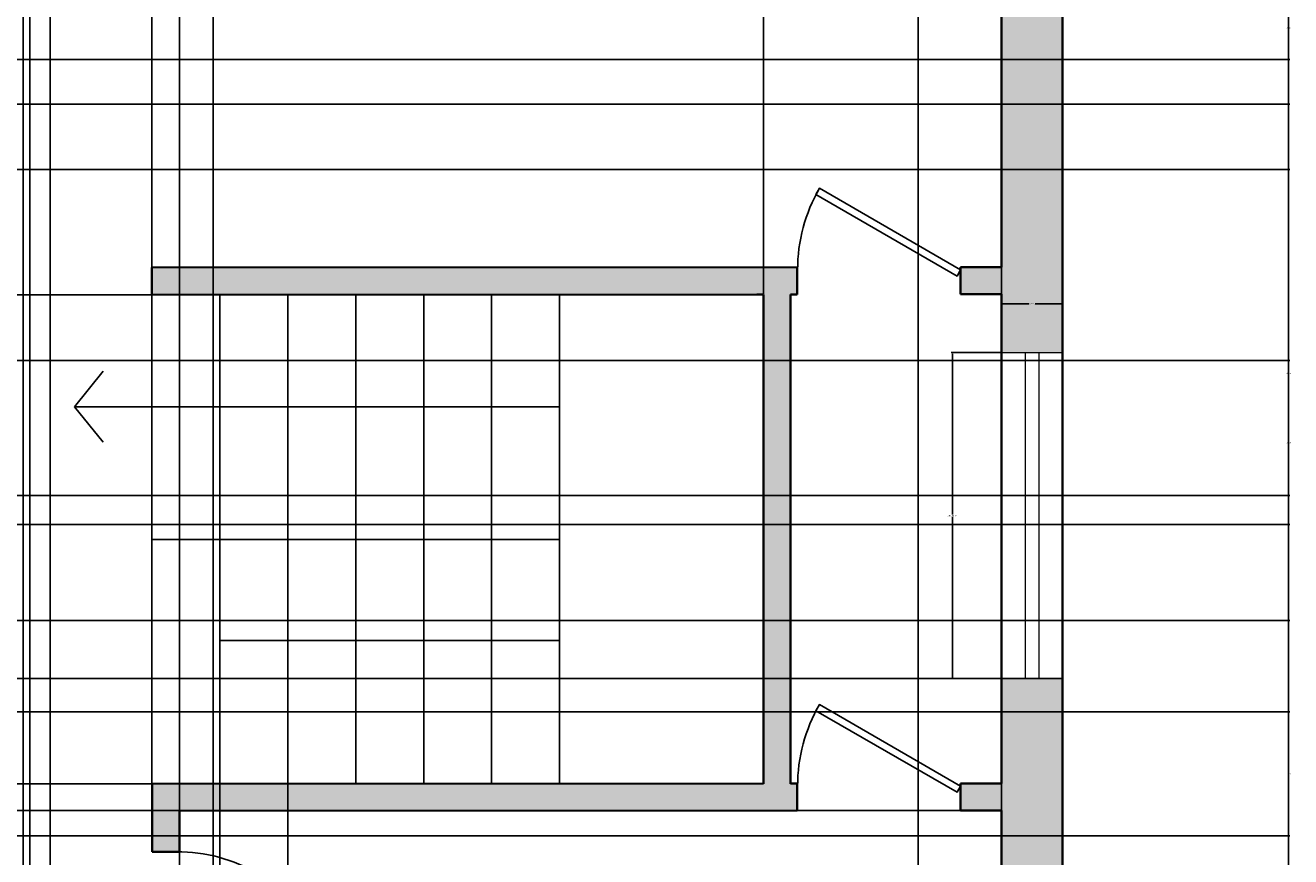
# Model space of a CAD drawing. Units: inches. Extents: x 1531 to 2263, y 2711 to 3216.
# Tile 10 of 12: x 2076 to 2262, y 2893 to 3015. Entities that reach past the tile are written whole.
import ezdxf

# ---------------------------------------------------------------- set-up
doc = ezdxf.new("R2010")
doc.units = ezdxf.units.IN
for name, color, linetype, lineweight in [('A-ANNO-DIMS', 2, 'Continuous', 18), ('A-DOOR', 3, 'Continuous', 25), ('A-FLOR-STRS', 7, 'Continuous', 25), ('A-GLAZ', 4, 'Continuous', 18), ('A-WALL', 7, 'Continuous', 35)]:
    doc.layers.add(name, color=color, linetype=linetype, lineweight=lineweight)
doc.layers.add('A-WALL-PATT', color=18, linetype='Continuous', lineweight=13, true_color=0x000000)
doc.styles.get("Standard").update_dxf_attribs({"font": 'arial.ttf'})
doc.dimstyles.get("Standard").update_dxf_attribs({"dimtxt": 0.18, "dimasz": 0.18, "dimexe": 0.18, "dimexo": 0.0625, "dimgap": 0.09, "dimtad": 0, "dimtih": 1, "dimtoh": 1, "dimdec": 4, "dimzin": 0, "dimdsep": 46, "dimtxsty": 'Standard', "dimcen": 0.09, "dimadec": 0, "dimazin": 0, "dimtfac": 1, "dimtdec": 4, "dimtofl": 0, "dimtmove": 0, "dimatfit": 3, "dimfxl": 1, "dimtolj": 1, "dimtzin": 0, "dimarcsym": 0})

# ---------------------------------------------------------------- blocks, each defined once
blk = doc.blocks.new('*U3')
for p, q in [((0, 0), (0, -6)), ((40, 0), (40, -6))]:
    blk.add_line(p, q)
blk.add_lwpolyline([(0, 0), (34.64, 20), (35.52, 18.48), (0.87, -1.52)], close=True)
blk.add_arc((0, 0), 40, 0, 30)
blk = doc.blocks.new('WIN-48IN')
for p, q in [((3.5, 48), (3.5, 0)), ((5.5, 48), (5.5, 0))]:
    blk.add_line(p, q)
for points in [[(0, 48), (9, 48)], [(9, 0), (0, 0)]]:
    blk.add_lwpolyline(points)
blk = doc.blocks.new('*D30')
at = {"layer": 'A-ANNO-DIMS', "color": 0, "lineweight": -2, "transparency": 16777216}
for p, q in [((2219.85, 2966.81), (2212.53, 2966.81)), ((2212.71, 2966.63), (2212.71, 2942.99)), ((2212.71, 2918.99), (2212.71, 2942.62)), ((2219.85, 2918.81), (2212.53, 2918.81))]:
    blk.add_line(p, q, dxfattribs=at)
at = {"layer": 'A-ANNO-DIMS', "color": 0, "transparency": 16777216}
for points in [[(2212.68, 2966.63), (2212.74, 2966.63), (2212.71, 2966.81)], [(2212.68, 2918.99), (2212.74, 2918.99), (2212.71, 2918.81)]]:
    blk.add_solid(points, dxfattribs=at)
at = {"layer": 'Defpoints', "color": 0, "transparency": 16777216}
for p in [(2212.71, 2966.81), (2219.91, 2966.81), (2219.91, 2918.81)]:
    blk.add_point(p, dxfattribs=at)
at = {"layer": 'A-ANNO-DIMS', "color": 0, "transparency": 16777216, "insert": (2212.71, 2942.81), "char_height": 0.18, "attachment_point": 5}
blk.add_mtext('\\A1;WDW 48 TYP.', dxfattribs=at)
blk = doc.blocks.new('*D31')
at = {"layer": 'A-ANNO-DIMS', "color": 0, "lineweight": -2, "transparency": 16777216}
for p, q in [((2219.91, 2966.87), (2219.91, 2974.19)), ((2220.09, 2974.01), (2223.95, 2974.01)), ((2228.73, 2974.01), (2224.87, 2974.01)), ((2228.91, 2966.87), (2228.91, 2974.19))]:
    blk.add_line(p, q, dxfattribs=at)
at = {"layer": 'A-ANNO-DIMS', "color": 0, "transparency": 16777216}
for points in [[(2220.09, 2974.04), (2220.09, 2973.98), (2219.91, 2974.01)], [(2228.73, 2974.04), (2228.73, 2973.98), (2228.91, 2974.01)]]:
    blk.add_solid(points, dxfattribs=at)
at = {"layer": 'Defpoints', "color": 0, "transparency": 16777216}
for p in [(2228.91, 2974.01), (2219.91, 2966.81), (2228.91, 2966.81)]:
    blk.add_point(p, dxfattribs=at)
at = {"layer": 'A-ANNO-DIMS', "color": 0, "transparency": 16777216, "insert": (2224.41, 2974.01), "char_height": 0.18, "attachment_point": 5}
blk.add_mtext('\\A1;9 TYP.', dxfattribs=at)
blk = doc.blocks.new('*D55')
at = {"layer": 'A-ANNO-DIMS', "color": 0, "lineweight": -2, "transparency": 16777216}
for p, q in [((2228.97, 3183.02), (2262.37, 3183.02)), ((2262.19, 3182.84), (2262.19, 2963.95)), ((2262.19, 2744.7), (2262.19, 2963.59)), ((2076.3, 2744.52), (2262.37, 2744.52))]:
    blk.add_line(p, q, dxfattribs=at)
at = {"layer": 'A-ANNO-DIMS', "color": 0, "transparency": 16777216}
for points in [[(2262.16, 3182.84), (2262.22, 3182.84), (2262.19, 3183.02)], [(2262.16, 2744.7), (2262.22, 2744.7), (2262.19, 2744.52)]]:
    blk.add_solid(points, dxfattribs=at)
at = {"layer": 'Defpoints', "color": 0, "transparency": 16777216}
for p in [(2228.91, 3183.02), (2076.24, 2744.52), (2262.19, 2744.52)]:
    blk.add_point(p, dxfattribs=at)
at = {"layer": 'A-ANNO-DIMS', "color": 0, "transparency": 16777216, "insert": (2262.19, 2963.77), "char_height": 0.18, "attachment_point": 5}
blk.add_mtext('\\A1;438.5', dxfattribs=at)
blk = doc.blocks.new('*D74')
at = {"layer": 'A-ANNO-DIMS', "color": 0, "lineweight": -2, "transparency": 16777216}
for p, q in [((2098.91, 2899.27), (2098.91, 2711.06)), ((2219.91, 2899.33), (2219.91, 2711.06)), ((2099.09, 2711.24), (2159.15, 2711.24)), ((2219.73, 2711.24), (2159.67, 2711.24))]:
    blk.add_line(p, q, dxfattribs=at)
at = {"layer": 'A-ANNO-DIMS', "color": 0, "transparency": 16777216}
for points in [[(2099.09, 2711.27), (2099.09, 2711.21), (2098.91, 2711.24)], [(2219.73, 2711.27), (2219.73, 2711.21), (2219.91, 2711.24)]]:
    blk.add_solid(points, dxfattribs=at)
at = {"layer": 'Defpoints', "color": 0, "transparency": 16777216}
for p in [(2098.91, 2899.33), (2219.91, 2899.4), (2219.91, 2711.24)]:
    blk.add_point(p, dxfattribs=at)
at = {"layer": 'A-ANNO-DIMS', "color": 0, "transparency": 16777216, "insert": (2159.41, 2711.24), "char_height": 0.18, "attachment_point": 5}
blk.add_mtext('\\A1;121', dxfattribs=at)
blk = doc.blocks.new('*D75')
at = {"layer": 'A-ANNO-DIMS', "color": 0, "lineweight": -2, "transparency": 16777216}
for p, q in [((2219.85, 2899.4), (1531.04, 2899.4)), ((1531.22, 2899.22), (1531.22, 2853.81)), ((1531.22, 2808.04), (1531.22, 2853.45)), ((2219.85, 2807.86), (1531.04, 2807.86))]:
    blk.add_line(p, q, dxfattribs=at)
at = {"layer": 'A-ANNO-DIMS', "color": 0, "transparency": 16777216}
for points in [[(1531.19, 2899.22), (1531.25, 2899.22), (1531.22, 2899.4)], [(1531.19, 2808.04), (1531.25, 2808.04), (1531.22, 2807.86)]]:
    blk.add_solid(points, dxfattribs=at)
at = {"layer": 'Defpoints', "color": 0, "transparency": 16777216}
for p in [(1531.22, 2899.4), (2219.91, 2899.4), (2219.91, 2807.86)]:
    blk.add_point(p, dxfattribs=at)
at = {"layer": 'A-ANNO-DIMS', "color": 0, "transparency": 16777216, "insert": (1531.22, 2853.63), "char_height": 0.18, "attachment_point": 5}
blk.add_mtext('\\A1;91.53', dxfattribs=at)
blk = doc.blocks.new('*D76')
at = {"layer": 'A-ANNO-DIMS', "color": 0, "lineweight": -2, "transparency": 16777216}
for p, q in [((2094.87, 2975.39), (2094.87, 3216.47)), ((2095.05, 3216.29), (2139.65, 3216.29)), ((2184.69, 3216.29), (2140.09, 3216.29)), ((2184.87, 2975.44), (2184.87, 3216.47))]:
    blk.add_line(p, q, dxfattribs=at)
at = {"layer": 'A-ANNO-DIMS', "color": 0, "transparency": 16777216}
for points in [[(2095.05, 3216.32), (2095.05, 3216.26), (2094.87, 3216.29)], [(2184.69, 3216.32), (2184.69, 3216.26), (2184.87, 3216.29)]]:
    blk.add_solid(points, dxfattribs=at)
at = {"layer": 'Defpoints', "color": 0, "transparency": 16777216}
for p in [(2184.87, 3216.29), (2094.87, 2975.33), (2184.87, 2975.38)]:
    blk.add_point(p, dxfattribs=at)
at = {"layer": 'A-ANNO-DIMS', "color": 0, "transparency": 16777216, "insert": (2139.87, 3216.29), "char_height": 0.18, "attachment_point": 5}
blk.add_mtext('\\A1;90', dxfattribs=at)
blk = doc.blocks.new('*D77')
at = {"layer": 'A-ANNO-DIMS', "color": 0, "lineweight": -2, "transparency": 16777216}
for p, q in [((2094.81, 2975.33), (1531.04, 2975.33)), ((1531.22, 2975.15), (1531.22, 2939.52)), ((1531.22, 2903.53), (1531.22, 2939.16)), ((2094.81, 2903.35), (1531.04, 2903.35))]:
    blk.add_line(p, q, dxfattribs=at)
at = {"layer": 'A-ANNO-DIMS', "color": 0, "transparency": 16777216}
for points in [[(1531.19, 2975.15), (1531.25, 2975.15), (1531.22, 2975.33)], [(1531.19, 2903.53), (1531.25, 2903.53), (1531.22, 2903.35)]]:
    blk.add_solid(points, dxfattribs=at)
at = {"layer": 'Defpoints', "color": 0, "transparency": 16777216}
for p in [(2094.87, 2975.33), (1531.22, 2903.35), (2094.87, 2903.35)]:
    blk.add_point(p, dxfattribs=at)
at = {"layer": 'A-ANNO-DIMS', "color": 0, "transparency": 16777216, "insert": (1531.22, 2939.34), "char_height": 0.18, "attachment_point": 5}
blk.add_mtext('\\A1;71.98', dxfattribs=at)
blk = doc.blocks.new('*D84')
at = {"layer": 'A-ANNO-DIMS', "color": 0, "lineweight": -2, "transparency": 16777216}
for p, q in [((2079.91, 3089.28), (2079.91, 2711.06)), ((2103.91, 3089.28), (2103.91, 2711.06)), ((2080.09, 2711.24), (2091.69, 2711.24)), ((2103.73, 2711.24), (2092.13, 2711.24))]:
    blk.add_line(p, q, dxfattribs=at)
at = {"layer": 'A-ANNO-DIMS', "color": 0, "transparency": 16777216}
for points in [[(2080.09, 2711.27), (2080.09, 2711.21), (2079.91, 2711.24)], [(2103.73, 2711.27), (2103.73, 2711.21), (2103.91, 2711.24)]]:
    blk.add_solid(points, dxfattribs=at)
at = {"layer": 'Defpoints', "color": 0, "transparency": 16777216}
for p in [(2079.91, 3089.34), (2103.91, 3089.34), (2103.91, 2711.24)]:
    blk.add_point(p, dxfattribs=at)
at = {"layer": 'A-ANNO-DIMS', "color": 0, "transparency": 16777216, "insert": (2091.91, 2711.24), "char_height": 0.18, "attachment_point": 5}
blk.add_mtext('\\A1;24', dxfattribs=at)
blk = doc.blocks.new('*D99')
at = {"layer": 'A-ANNO-DIMS', "color": 0, "lineweight": -2, "transparency": 16777216}
for p, q in [((1894.62, 3003.38), (2262.37, 3003.38)), ((2262.19, 3003.2), (2262.19, 2965.56)), ((2262.19, 2927.56), (2262.19, 2965.19)), ((1894.62, 2927.38), (2262.37, 2927.38))]:
    blk.add_line(p, q, dxfattribs=at)
at = {"layer": 'A-ANNO-DIMS', "color": 0, "transparency": 16777216}
for points in [[(2262.16, 3003.2), (2262.22, 3003.2), (2262.19, 3003.38)], [(2262.16, 2927.56), (2262.22, 2927.56), (2262.19, 2927.38)]]:
    blk.add_solid(points, dxfattribs=at)
at = {"layer": 'Defpoints', "color": 0, "transparency": 16777216}
for p in [(1894.55, 3003.38), (1894.55, 2927.38), (2262.19, 2927.38)]:
    blk.add_point(p, dxfattribs=at)
at = {"layer": 'A-ANNO-DIMS', "color": 0, "transparency": 16777216, "insert": (2262.19, 2965.38), "char_height": 0.18, "attachment_point": 5}
blk.add_mtext('\\A1;76', dxfattribs=at)
blk = doc.blocks.new('*D101')
at = {"layer": 'A-ANNO-DIMS', "color": 0, "lineweight": -2, "transparency": 16777216}
for p, q in [((2228.85, 2918.81), (1531.04, 2918.81)), ((1531.22, 2918.63), (1531.22, 2897.08)), ((1531.22, 2875.18), (1531.22, 2896.72)), ((2228.85, 2875), (1531.04, 2875))]:
    blk.add_line(p, q, dxfattribs=at)
at = {"layer": 'A-ANNO-DIMS', "color": 0, "transparency": 16777216}
for points in [[(1531.19, 2918.63), (1531.25, 2918.63), (1531.22, 2918.81)], [(1531.19, 2875.18), (1531.25, 2875.18), (1531.22, 2875)]]:
    blk.add_solid(points, dxfattribs=at)
at = {"layer": 'Defpoints', "color": 0, "transparency": 16777216}
for p in [(2228.91, 2918.81), (1531.22, 2875), (2228.91, 2875)]:
    blk.add_point(p, dxfattribs=at)
at = {"layer": 'A-ANNO-DIMS', "color": 0, "transparency": 16777216, "insert": (1531.22, 2896.9), "char_height": 0.18, "attachment_point": 5}
blk.add_mtext('\\A1;43.81', dxfattribs=at)
blk = doc.blocks.new('*D105')
at = {"layer": 'A-ANNO-DIMS', "color": 0, "lineweight": -2, "transparency": 16777216}
for p, q in [((2104.87, 2975.27), (2104.87, 2711.06)), ((2114.87, 2975.27), (2114.87, 2711.06)), ((2105.05, 2711.24), (2109.66, 2711.24)), ((2114.69, 2711.24), (2110.08, 2711.24))]:
    blk.add_line(p, q, dxfattribs=at)
at = {"layer": 'A-ANNO-DIMS', "color": 0, "transparency": 16777216}
for points in [[(2105.05, 2711.27), (2105.05, 2711.21), (2104.87, 2711.24)], [(2114.69, 2711.27), (2114.69, 2711.21), (2114.87, 2711.24)]]:
    blk.add_solid(points, dxfattribs=at)
at = {"layer": 'Defpoints', "color": 0, "transparency": 16777216}
for p in [(2104.87, 2975.33), (2114.87, 2975.33), (2114.87, 2711.24)]:
    blk.add_point(p, dxfattribs=at)
at = {"layer": 'A-ANNO-DIMS', "color": 0, "transparency": 16777216, "insert": (2109.87, 2711.24), "char_height": 0.18, "attachment_point": 5}
blk.add_mtext('\\A1;10', dxfattribs=at)
blk = doc.blocks.new('*D112')
at = {"layer": 'A-ANNO-DIMS', "color": 0, "lineweight": -2, "transparency": 16777216}
for p, q in [((1721.97, 3009.94), (2262.37, 3009.94)), ((2262.19, 3009.76), (2262.19, 2962.12)), ((2262.19, 2914.12), (2262.19, 2961.76)), ((1721.97, 2913.94), (2262.37, 2913.94))]:
    blk.add_line(p, q, dxfattribs=at)
at = {"layer": 'A-ANNO-DIMS', "color": 0, "transparency": 16777216}
for points in [[(2262.16, 3009.76), (2262.22, 3009.76), (2262.19, 3009.94)], [(2262.16, 2914.12), (2262.22, 2914.12), (2262.19, 2913.94)]]:
    blk.add_solid(points, dxfattribs=at)
at = {"layer": 'Defpoints', "color": 0, "transparency": 16777216}
for p in [(1721.91, 3009.94), (1721.91, 2913.94), (2262.19, 2913.94)]:
    blk.add_point(p, dxfattribs=at)
at = {"layer": 'A-ANNO-DIMS', "color": 0, "transparency": 16777216, "insert": (2262.19, 2961.94), "char_height": 0.18, "attachment_point": 5}
blk.add_mtext('\\A1;96', dxfattribs=at)
blk = doc.blocks.new('*D114')
at = {"layer": 'A-ANNO-DIMS', "color": 0, "lineweight": -2, "transparency": 16777216}
for p, q in [((1577.97, 2913.94), (2262.37, 2913.94)), ((2262.19, 2913.76), (2262.19, 2904.99)), ((2262.19, 2895.86), (2262.19, 2904.63)), ((1577.97, 2895.68), (2262.37, 2895.68))]:
    blk.add_line(p, q, dxfattribs=at)
at = {"layer": 'A-ANNO-DIMS', "color": 0, "transparency": 16777216}
for points in [[(2262.16, 2913.76), (2262.22, 2913.76), (2262.19, 2913.94)], [(2262.16, 2895.86), (2262.22, 2895.86), (2262.19, 2895.68)]]:
    blk.add_solid(points, dxfattribs=at)
at = {"layer": 'Defpoints', "color": 0, "transparency": 16777216}
for p in [(1577.91, 2913.94), (1577.91, 2895.68), (2262.19, 2895.68)]:
    blk.add_point(p, dxfattribs=at)
at = {"layer": 'A-ANNO-DIMS', "color": 0, "transparency": 16777216, "insert": (2262.19, 2904.81), "char_height": 0.18, "attachment_point": 5}
blk.add_mtext('\\A1;18.26', dxfattribs=at)
blk = doc.blocks.new('*D116')
at = {"layer": 'A-ANNO-DIMS', "color": 0, "lineweight": -2, "transparency": 16777216}
for p, q in [((1899.97, 3025.85), (2262.37, 3025.85)), ((2262.19, 3025.67), (2262.19, 3014.79)), ((2262.19, 3003.56), (2262.19, 3014.43)), ((1894.62, 3003.38), (2262.37, 3003.38))]:
    blk.add_line(p, q, dxfattribs=at)
at = {"layer": 'A-ANNO-DIMS', "color": 0, "transparency": 16777216}
for points in [[(2262.16, 3025.67), (2262.22, 3025.67), (2262.19, 3025.85)], [(2262.16, 3003.56), (2262.22, 3003.56), (2262.19, 3003.38)]]:
    blk.add_solid(points, dxfattribs=at)
at = {"layer": 'Defpoints', "color": 0, "transparency": 16777216}
for p in [(1899.91, 3025.85), (1894.55, 3003.38), (2262.19, 3003.38)]:
    blk.add_point(p, dxfattribs=at)
at = {"layer": 'A-ANNO-DIMS', "color": 0, "transparency": 16777216, "insert": (2262.19, 3014.61), "char_height": 0.18, "attachment_point": 5}
blk.add_mtext('\\A1;22.47', dxfattribs=at)
blk = doc.blocks.new('*D118')
at = {"layer": 'A-ANNO-DIMS', "color": 0, "lineweight": -2, "transparency": 16777216}
for p, q in [((1851.5, 2965.63), (2262.37, 2965.63)), ((2262.19, 2965.45), (2262.19, 2953.74)), ((2262.19, 2941.67), (2262.19, 2953.38)), ((1851.5, 2941.49), (2262.37, 2941.49))]:
    blk.add_line(p, q, dxfattribs=at)
at = {"layer": 'A-ANNO-DIMS', "color": 0, "transparency": 16777216}
for points in [[(2262.16, 2965.45), (2262.22, 2965.45), (2262.19, 2965.63)], [(2262.16, 2941.67), (2262.22, 2941.67), (2262.19, 2941.49)]]:
    blk.add_solid(points, dxfattribs=at)
at = {"layer": 'Defpoints', "color": 0, "transparency": 16777216}
for p in [(1851.44, 2965.63), (1851.44, 2941.49), (2262.19, 2941.49)]:
    blk.add_point(p, dxfattribs=at)
at = {"layer": 'A-ANNO-DIMS', "color": 0, "transparency": 16777216, "insert": (2262.19, 2953.56), "char_height": 0.18, "attachment_point": 5}
blk.add_mtext('\\A1;24.14', dxfattribs=at)
blk = doc.blocks.new('*D120')
at = {"layer": 'A-ANNO-DIMS', "color": 0, "lineweight": -2, "transparency": 16777216}
for p, q in [((1797.97, 2993.76), (2262.37, 2993.76)), ((2262.19, 2993.58), (2262.19, 2969.95)), ((2262.19, 2945.94), (2262.19, 2969.58)), ((1797.97, 2945.76), (2262.37, 2945.76))]:
    blk.add_line(p, q, dxfattribs=at)
at = {"layer": 'A-ANNO-DIMS', "color": 0, "transparency": 16777216}
for points in [[(2262.16, 2993.58), (2262.22, 2993.58), (2262.19, 2993.76)], [(2262.16, 2945.94), (2262.22, 2945.94), (2262.19, 2945.76)]]:
    blk.add_solid(points, dxfattribs=at)
at = {"layer": 'Defpoints', "color": 0, "transparency": 16777216}
for p in [(1797.91, 2993.76), (2262.19, 2993.76), (1797.91, 2945.76)]:
    blk.add_point(p, dxfattribs=at)
at = {"layer": 'A-ANNO-DIMS', "color": 0, "transparency": 16777216, "insert": (2262.19, 2969.76), "char_height": 0.18, "attachment_point": 5}
blk.add_mtext('\\A1;48', dxfattribs=at)
blk = doc.blocks.new('*D121')
at = {"layer": 'A-ANNO-DIMS', "color": 0, "lineweight": -2, "transparency": 16777216}
for p, q in [((2052, 2979.08), (2052, 3216.47)), ((2052.18, 3216.29), (2073.04, 3216.29)), ((2094.69, 3216.29), (2073.83, 3216.29)), ((2094.87, 2979.39), (2094.87, 3216.47))]:
    blk.add_line(p, q, dxfattribs=at)
at = {"layer": 'A-ANNO-DIMS', "color": 0, "transparency": 16777216}
for points in [[(2052.18, 3216.32), (2052.18, 3216.26), (2052, 3216.29)], [(2094.69, 3216.32), (2094.69, 3216.26), (2094.87, 3216.29)]]:
    blk.add_solid(points, dxfattribs=at)
at = {"layer": 'Defpoints', "color": 0, "transparency": 16777216}
for p in [(2094.87, 3216.29), (2052, 2979.01), (2094.87, 2979.33)]:
    blk.add_point(p, dxfattribs=at)
at = {"layer": 'A-ANNO-DIMS', "color": 0, "transparency": 16777216, "insert": (2073.43, 3216.29), "char_height": 0.18, "attachment_point": 5}
blk.add_mtext('\\A1;42.87', dxfattribs=at)
blk = doc.blocks.new('*D123')
at = {"layer": 'A-ANNO-DIMS', "color": 0, "lineweight": -2, "transparency": 16777216}
for p, q in [((2207.66, 3152.42), (2207.66, 2711.06)), ((2219.92, 3149.95), (2219.92, 2711.06)), ((2207.84, 2711.24), (2213.41, 2711.24)), ((2219.74, 2711.24), (2214.18, 2711.24))]:
    blk.add_line(p, q, dxfattribs=at)
at = {"layer": 'A-ANNO-DIMS', "color": 0, "transparency": 16777216}
for points in [[(2207.84, 2711.27), (2207.84, 2711.21), (2207.66, 2711.24)], [(2219.74, 2711.27), (2219.74, 2711.21), (2219.92, 2711.24)]]:
    blk.add_solid(points, dxfattribs=at)
at = {"layer": 'Defpoints', "color": 0, "transparency": 16777216}
for p in [(2207.66, 3152.48), (2219.92, 3150.02), (2207.66, 2711.24)]:
    blk.add_point(p, dxfattribs=at)
at = {"layer": 'A-ANNO-DIMS', "color": 0, "transparency": 16777216, "insert": (2213.79, 2711.24), "char_height": 0.18, "attachment_point": 5}
blk.add_mtext('\\A1;12.26', dxfattribs=at)
blk = doc.blocks.new('*D124')
at = {"layer": 'A-ANNO-DIMS', "color": 0, "lineweight": -2, "transparency": 16777216}
for p, q in [((2076.91, 2862.01), (2076.91, 3216.47)), ((2077.09, 3216.29), (2087.69, 3216.29)), ((2098.73, 3216.29), (2088.13, 3216.29)), ((2098.91, 2862.01), (2098.91, 3216.47))]:
    blk.add_line(p, q, dxfattribs=at)
at = {"layer": 'A-ANNO-DIMS', "color": 0, "transparency": 16777216}
for points in [[(2077.09, 3216.32), (2077.09, 3216.26), (2076.91, 3216.29)], [(2098.73, 3216.32), (2098.73, 3216.26), (2098.91, 3216.29)]]:
    blk.add_solid(points, dxfattribs=at)
at = {"layer": 'Defpoints', "color": 0, "transparency": 16777216}
for p in [(2076.91, 3216.29), (2076.91, 2861.95), (2098.91, 2861.95)]:
    blk.add_point(p, dxfattribs=at)
at = {"layer": 'A-ANNO-DIMS', "color": 0, "transparency": 16777216, "insert": (2087.91, 3216.29), "char_height": 0.18, "attachment_point": 5}
blk.add_mtext('\\A1;22', dxfattribs=at)
blk = doc.blocks.new('*D130')
at = {"layer": 'A-ANNO-DIMS', "color": 0, "lineweight": -2, "transparency": 16777216}
for p, q in [((2075.91, 3029.88), (2075.91, 2711.06)), ((2079.91, 3025.88), (2079.91, 2711.06)), ((2076.09, 2711.24), (2077.76, 2711.24)), ((2079.73, 2711.24), (2078.06, 2711.24))]:
    blk.add_line(p, q, dxfattribs=at)
at = {"layer": 'A-ANNO-DIMS', "color": 0, "transparency": 16777216}
for points in [[(2076.09, 2711.27), (2076.09, 2711.21), (2075.91, 2711.24)], [(2079.73, 2711.27), (2079.73, 2711.21), (2079.91, 2711.24)]]:
    blk.add_solid(points, dxfattribs=at)
at = {"layer": 'Defpoints', "color": 0, "transparency": 16777216}
for p in [(2075.91, 3029.94), (2079.91, 3025.94), (2075.91, 2711.24)]:
    blk.add_point(p, dxfattribs=at)
at = {"layer": 'A-ANNO-DIMS', "color": 0, "transparency": 16777216, "insert": (2077.91, 2711.24), "char_height": 0.18, "attachment_point": 5}
blk.add_mtext('\\A1;4', dxfattribs=at)

msp = doc.modelspace()

# ---------------------------------------------------------------- hatches: boundary and pattern name
at = {"layer": 'A-WALL-PATT'}
h = msp.add_hatch(color=256, dxfattribs=at)
h.dxf.hatch_style = 1
h.paths.add_polyline_path([(2228.9101, 3065.4897), (2219.9101, 3065.4897), (2219.9101, 3026.0153), (2219.9101, 2979.3969), (2213.9101, 2979.3937), (2213.9101, 2975.3937), (2219.9101, 2975.3969), (2219.9101, 2966.8056), (2228.9101, 2966.8056)])
h = msp.add_hatch(color=256, dxfattribs=at)
h.dxf.hatch_style = 1
h.paths.add_polyline_path([(2189.8725, 2903.3811), (2188.8725, 2903.3806), (2188.8725, 2975.3806), (2189.8725, 2975.3811), (2189.8725, 2979.3811), (2094.8704, 2979.3315), (2094.8725, 2975.3315), (2183.9101, 2975.378), (2184.8725, 2975.3785), (2184.8725, 2903.3785), (2094.9101, 2903.3315), (2094.9101, 2895.9499), (2094.9101, 2893.3336), (2098.9101, 2893.3336), (2098.9101, 2899.3336), (2189.8725, 2899.3811)])
h = msp.add_hatch(color=256, dxfattribs=at)
h.dxf.hatch_style = 1
h.paths.add_polyline_path([(2228.9101, 2918.8056), (2219.9101, 2918.8056), (2219.9101, 2903.3968), (2213.9101, 2903.3937), (2213.9101, 2899.3968), (2219.9101, 2899.3968), (2219.9101, 2874.9957), (2228.9101, 2874.9957)])

# ---------------------------------------------------------------- linework, layer by layer
at = {"layer": 'A-FLOR-STRS'}
for p, q in [((2094.8725, 2975.3315), (2094.8725, 2903.3482)), ((2104.8725, 2975.3315), (2104.8725, 2903.3482)), ((2114.8725, 2975.3315), (2114.8725, 2903.3482)), ((2124.8725, 2975.3315), (2124.8725, 2903.3482)), ((2134.8725, 2975.3315), (2134.8725, 2903.3482)), ((2144.8725, 2975.3315), (2144.8725, 2903.3482)), ((2154.8725, 2975.3315), (2154.8725, 2903.3482)), ((2083.4995, 2958.8476), (2087.6936, 2964.0848)), ((2154.8725, 2958.8476), (2083.4995, 2958.8476)), ((2083.4995, 2958.8476), (2087.6936, 2953.6103)), ((2154.8725, 2939.3158), (2094.8725, 2939.2844)), ((2104.8725, 2924.4377), (2154.8725, 2924.4377)), ((2104.9101, 2903.3367), (2104.9101, 2903.3315)), ((2114.9101, 2903.3419), (2114.9101, 2903.3315)), ((2124.9101, 2903.3472), (2124.9101, 2903.3315)), ((2134.9101, 2903.3524), (2134.9101, 2903.3315)), ((2144.9101, 2903.3576), (2144.9101, 2903.3315)), ((2154.9101, 2903.3629), (2154.9101, 2903.3315)), ((2164.8725, 2903.3681), (2164.8725, 2903.3482)), ((2164.9101, 2903.3681), (2164.9101, 2903.3315)), ((2174.8725, 2903.3733), (2174.8725, 2903.3482)), ((2174.9101, 2903.3733), (2174.9101, 2903.3315))]:
    msp.add_line(p, q, dxfattribs=at)
at = {"layer": 'A-WALL'}
for p, q in [((2219.9101, 3026.0153), (2219.9101, 2979.3969)), ((2189.8725, 2979.3811), (2094.8704, 2979.3315)), ((2094.8704, 2979.3315), (2094.8725, 2975.3315)), ((2189.8725, 2975.3806), (2189.8725, 2979.3811)), ((2219.9101, 2979.3969), (2213.9101, 2979.3937)), ((2213.9101, 2979.3969), (2213.9101, 2975.3937)), ((2183.9101, 2975.378), (2094.8725, 2975.3315)), ((2183.9101, 2975.378), (2184.8725, 2975.3785)), ((2184.8725, 2975.3785), (2184.8725, 2903.3482)), ((2189.8725, 2975.3811), (2188.8725, 2975.3806)), ((2188.8725, 2975.3806), (2188.8725, 2903.3482)), ((2219.9101, 2975.3969), (2213.9101, 2975.3937)), ((2219.9101, 2975.3969), (2219.9101, 2903.3968)), ((2184.8725, 2903.3785), (2094.9101, 2903.3315)), ((2094.9101, 2895.9499), (2094.9101, 2903.3315)), ((2189.8725, 2903.3811), (2188.8725, 2903.3806)), ((2189.8725, 2903.3811), (2189.8725, 2899.3806)), ((2219.9101, 2903.3968), (2213.9101, 2903.3937)), ((2213.9101, 2903.3937), (2213.9101, 2899.3968)), ((2189.8725, 2899.3811), (2098.9101, 2899.3336)), ((2098.9101, 2893.3336), (2098.9101, 2899.3336)), ((2213.9101, 2899.3968), (2219.9101, 2899.3968)), ((2219.9101, 2899.3968), (2219.9101, 2807.8631)), ((2219.9101, 2899.3968), (2219.9101, 2896.0153)), ((2094.9101, 2895.9499), (2094.9101, 2893.3336)), ((2098.9101, 2893.3336), (2094.9101, 2893.3336))]:
    msp.add_line(p, q, dxfattribs=at)
msp.add_lwpolyline([(1933.9101, 2762.8657), (1568.9111, 2762.6748), (1568.9111, 3182.6749), (2228.9101, 3183.02), (2228.9101, 2798.8631)], dxfattribs=at)

# ---------------------------------------------------------------- block references
at = {"layer": 'A-DOOR', "xscale": -0.6, "yscale": 0.6, "zscale": 0.6}
for p in [(2213.9101, 2978.9937), (2213.9101, 2902.9968)]:
    msp.add_blockref('*U3', p, dxfattribs=at)
at = {"layer": 'A-DOOR', "xscale": -0.6, "yscale": 0.6, "zscale": 0.6, "rotation": 270}
msp.add_blockref('*U3', (2098.5101, 2869.3336), dxfattribs=at)
at = {"layer": 'A-GLAZ'}
msp.add_blockref('WIN-48IN', (2219.9101, 2918.8061), dxfattribs=at)

# ---------------------------------------------------------------- dimensions: what is measured, and where the dimension line sits
at = {"layer": 'A-ANNO-DIMS'}
for base, p1, p2, override, picture, middle in [((2094.8704, 3216.295), (2051.9983, 2979.0128), (2094.8704, 2979.3315), {"dimdec": 2, "dimlfac": 1, "dimrnd": 0, "dimzin": 0, "dimdsep": 46, "dimlunit": 2}, '*D121', (2073.4343, 3216.295)), ((2076.9101, 3216.295), (2098.9101, 2861.9499), (2076.9101, 2861.9499), {"dimdec": 0, "dimlfac": 1, "dimrnd": 0, "dimzin": 0, "dimdsep": 46, "dimlunit": 2}, '*D124', (2087.9101, 3216.295)), ((2184.8725, 3216.295), (2094.8725, 2975.3315), (2184.8725, 2975.3785), {"dimdec": 0, "dimlfac": 1, "dimrnd": 0, "dimzin": 0, "dimdsep": 46, "dimlunit": 2}, '*D76', (2139.8725, 3216.295)), ((2207.6621, 2711.2407), (2219.9227, 3150.0153), (2207.6621, 3152.4778), {"dimdec": 2, "dimlfac": 1, "dimrnd": 0, "dimzin": 0, "dimdsep": 46, "dimlunit": 2}, '*D123', (2213.7924, 2711.2407)), ((2103.9101, 2711.2407), (2079.9101, 3089.343), (2103.9101, 3089.343), {"dimdec": 0, "dimlfac": 1, "dimrnd": 0, "dimzin": 0, "dimdsep": 46, "dimlunit": 2}, '*D84', (2091.9101, 2711.2407)), ((2075.9101, 2711.2407), (2079.9101, 3025.9421), (2075.9101, 3029.94), {"dimdec": 0, "dimlfac": 1, "dimrnd": 0, "dimzin": 0, "dimdsep": 46, "dimlunit": 2}, '*D130', (2077.9101, 2711.2407)), ((2114.8725, 2711.2407), (2104.8725, 2975.3315), (2114.8725, 2975.3315), {"dimdec": 0, "dimlfac": 1, "dimrnd": 0, "dimzin": 0, "dimdsep": 46, "dimlunit": 2}, '*D105', (2109.8725, 2711.2407)), ((2219.9101, 2711.2407), (2098.9101, 2899.3336), (2219.9101, 2899.3968), {"dimdec": 0, "dimlfac": 1, "dimrnd": 0, "dimzin": 0, "dimdsep": 46, "dimlunit": 2}, '*D74', (2159.4101, 2711.2407))]:
    dim = msp.add_linear_dim(base=base, p1=p1, p2=p2, dimstyle='Standard', override=override, dxfattribs=at)
    dim.commit()
    dim.dimension.update_dxf_attribs({"geometry": picture, "text_midpoint": middle})
for base, p1, p2, override, picture, middle in [((2262.1851, 2744.5157), (2228.9101, 3183.02), (2076.2365, 2744.5157), {"dimdec": 1, "dimlfac": 1, "dimrnd": 0, "dimzin": 0, "dimdsep": 46, "dimlunit": 2}, '*D55', (2262.1851, 2963.7678)), ((2262.1851, 3003.376), (1899.9101, 3025.8479), (1894.5532, 3003.376), {"dimdec": 2, "dimlfac": 1, "dimrnd": 0, "dimzin": 0, "dimdsep": 46, "dimlunit": 2}, '*D116', (2262.1851, 3014.6119)), ((2262.1851, 2913.9378), (1721.9111, 3009.9378), (1721.9111, 2913.9378), {"dimdec": 0, "dimlfac": 1, "dimrnd": 0, "dimzin": 0, "dimdsep": 46, "dimlunit": 2}, '*D112', (2262.1851, 2961.9378)), ((2262.1851, 2927.376), (1894.5532, 3003.376), (1894.5532, 2927.376), {"dimdec": 0, "dimlfac": 1, "dimrnd": 0, "dimzin": 0, "dimdsep": 46, "dimlunit": 2}, '*D99', (2262.1851, 2965.376)), ((2262.1851, 2993.7637), (1797.9101, 2945.7637), (1797.9101, 2993.7637), {"dimdec": 0, "dimlfac": 1, "dimrnd": 0, "dimzin": 0, "dimdsep": 46, "dimlunit": 2}, '*D120', (2262.1851, 2969.7637)), ((1531.2212, 2903.3482), (2094.8725, 2975.3315), (2094.8725, 2903.3482), {"dimdec": 2, "dimlfac": 1, "dimrnd": 0, "dimzin": 0, "dimdsep": 46, "dimlunit": 2}, '*D77', (1531.2212, 2939.3398)), ((2262.1851, 2941.4913), (1851.4391, 2965.6329), (1851.4391, 2941.4913), {"dimdec": 2, "dimlfac": 1, "dimrnd": 0, "dimzin": 0, "dimdsep": 46, "dimlunit": 2}, '*D118', (2262.1851, 2953.5621)), ((1531.2212, 2874.9957), (2228.9101, 2918.8056), (2228.9101, 2874.9957), {"dimdec": 2, "dimlfac": 1, "dimrnd": 0, "dimzin": 0, "dimdsep": 46, "dimlunit": 2}, '*D101', (1531.2212, 2896.9007)), ((2262.1851, 2895.6796), (1577.9111, 2913.9378), (1577.9111, 2895.6796), {"dimdec": 2, "dimlfac": 1, "dimrnd": 0, "dimzin": 0, "dimdsep": 46, "dimlunit": 2}, '*D114', (2262.1851, 2904.8087)), ((1531.2212, 2899.3968), (2219.9101, 2807.8631), (2219.9101, 2899.3968), {"dimdec": 2, "dimlfac": 1, "dimrnd": 0, "dimzin": 0, "dimdsep": 46, "dimlunit": 2}, '*D75', (1531.2212, 2853.63))]:
    dim = msp.add_linear_dim(base=base, p1=p1, p2=p2, angle=90, dimstyle='Standard', override=override, dxfattribs=at)
    dim.commit()
    dim.dimension.update_dxf_attribs({"geometry": picture, "text_midpoint": middle})
dim = msp.add_linear_dim(base=(2228.9101, 2974.0056), p1=(2219.9101, 2966.8056), p2=(2228.9101, 2966.8056), text='<> TYP.', dimstyle='Standard', override={"dimdec": 0, "dimlfac": 1, "dimrnd": 0, "dimzin": 0, "dimdsep": 46, "dimlunit": 2}, dxfattribs=at)
dim.commit()
dim.dimension.update_dxf_attribs({"geometry": '*D31', "text_midpoint": (2224.4101, 2974.0056)})
dim = msp.add_linear_dim(base=(2212.7101, 2966.8056), p1=(2219.9101, 2918.8056), p2=(2219.9101, 2966.8056), angle=90, text='WDW <> TYP.', dimstyle='Standard', override={"dimdec": 0, "dimlfac": 1, "dimrnd": 0, "dimzin": 0, "dimdsep": 46, "dimlunit": 2}, dxfattribs=at)
dim.commit()
dim.dimension.update_dxf_attribs({"geometry": '*D30', "text_midpoint": (2212.7101, 2942.8056)})

doc.saveas('drawing.dxf')
